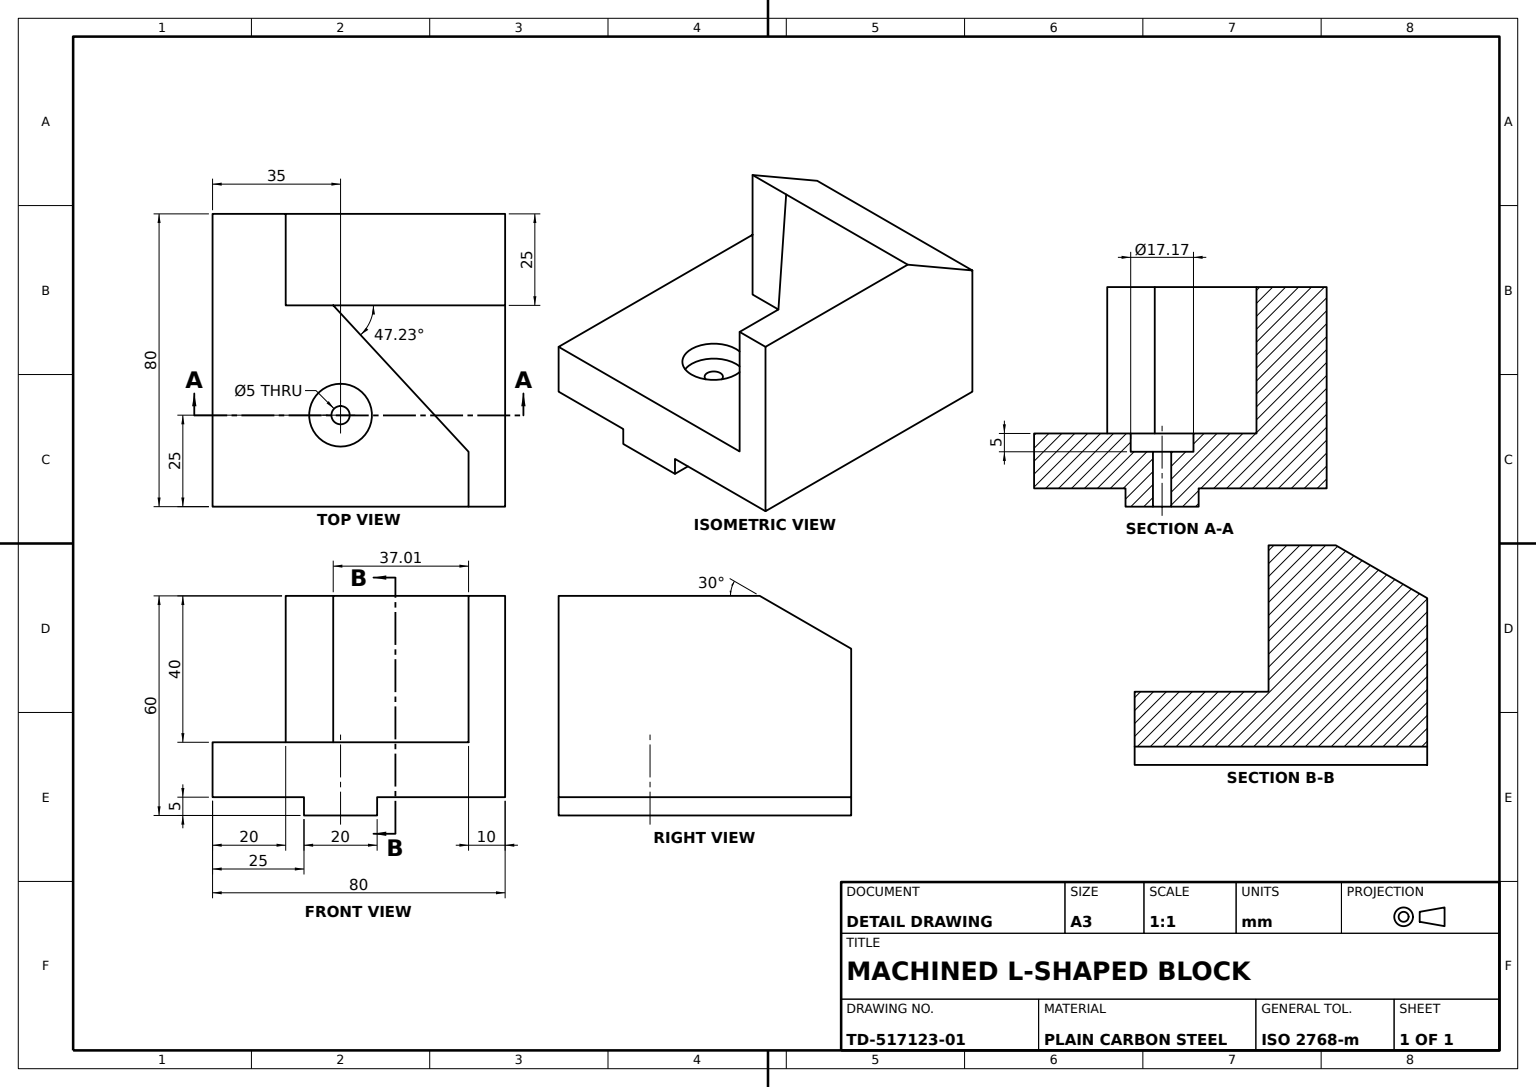
SolidWorks part; units mm, degrees
material "Plain Carbon Steel"
ref_plane "Front Plane" through (0, 0, 0) normal (0, 0, 1) x (1, 0, 0)
ref_plane "Top Plane" through (0, 0, 0) normal (0, 1, 0) x (1, 0, 0)
ref_plane "Right Plane" through (0, 0, 0) normal (1, 0, 0) x (0, 0, -1)
sketch "Base Profile Sketch" plane through (0, 0, 0) normal (0, 0, 1) x (1, 0, 0)
  line L15 (-40, -10) -> (40, -10)
  line L16 (-40, -10) -> (-40, 10)
  line L17 (-40, 10) -> (40, 10)
  line L18 (40, -10) -> (40, 10)
  line L19 (-40, -10) -> (40, 10) construction
  line L20 (-40, 10) -> (40, -10) construction
  point P0 (0, 0)
  dimension "D1" = 80
  dimension "D2" = 20
extrude "Base Block" add sketch "Base Profile Sketch" along normal blind 80
sketch "Underside Slot Sketch" plane through (0, 0, 80) normal (0, 0, 1) x (1, 0, 0)
  line L0 (-40, -5) -> (-40, -10)
  line L1 (-40, 10) -> (-40, -10) construction
  line L2 (-40, -5) -> (-15, -5)
  line L3 (-15, -5) -> (-15, -10)
  line L4 (-40, -10) -> (40, -10) construction
  line L5 (-15, -10) -> (5, -10)
  line L6 (5, -10) -> (5, -5)
  line L7 (5, -5) -> (40, -5)
  line L8 (40, -10) -> (40, 10) construction
  line L9 (5, -10) -> (40, -10)
  line L10 (40, -10) -> (40, -5)
  line L11 (-40, -10) -> (-15, -10)
  line L12 (40, 10) -> (-40, 10) construction
  dimension "D1" = 15
  dimension "D2" = 25
  dimension "D3" = 20
extrude "Underside Slot" cut sketch "Underside Slot Sketch" against normal blind 80 contours L3 L2 L0 L11 | L6 L7 L10 L9
sketch "Upright Wall Sketch" plane through (0, 10, 0) normal (0, 1, 0) x (1, 0, 0)
  line L1 (30, -80) -> (40, -80)
  line L2 (30, -80) -> (30, 0)
  line L3 (30, -80) -> (30, 0)
  line L4 (40, 0) -> (40, -80)
  line L5 (30, 0) -> (40, 0)
  dimension "D1" = 10
extrude "Upright Wall" add sketch "Upright Wall Sketch" along normal blind 40 contours L3 L5 L4 L1
sketch "Side Block Sketch" plane through (0, 10, 0) normal (0, 1, 0) x (1, 0, 0)
  line L0 (-20, 0) -> (-20, -25)
  line L1 (30, 0) -> (-40, 0) construction
  line L3 (30, -80) -> (30, 0) construction
  line L5 (30, -80) -> (30, 0) construction
  line L6 (-20, 0) -> (30, 0)
  line L7 (30, 0) -> (30, -65)
  line L8 (-7.0066, -25) -> (-20, -25)
  line L9 (-7.0066, -25) -> (30, -65)
  dimension "D1" = 25
  dimension "D2" = 37.0066
  dimension "D3" = 50
  dimension "D4" = 15
extrude "Side Block" add sketch "Side Block Sketch" along normal blind 40
chamfer "Wall Chamfer 25x30deg" distance 25 angle 30 1 edges at (10, 50, 0)
sketch "Counterbore Sketch" plane through (0, 10, 0) normal (0, 1, 0) x (1, 0, 0)
  line L0 (-40, -80) -> (-40, 0) construction
  line L1 (30, -80) -> (-40, -80) construction
  circle A0 centre (-5, -55) radius 8.5839
  dimension "D3" = 17.1678
  dimension "D1" = 35
  dimension "D2" = 25
extrude "Counterbore Recess" cut sketch "Counterbore Sketch" against normal blind 5 contours A0
sketch "Hole Sketch" plane through (0, 5, 0) normal (0, 1, 0) x (1, 0, 0)
  circle A0 centre (-5, -55) radius 2.5
  dimension "D1" = 5
extrude "Hole Dia5" cut sketch "Hole Sketch" against normal blind 22 contours A0
